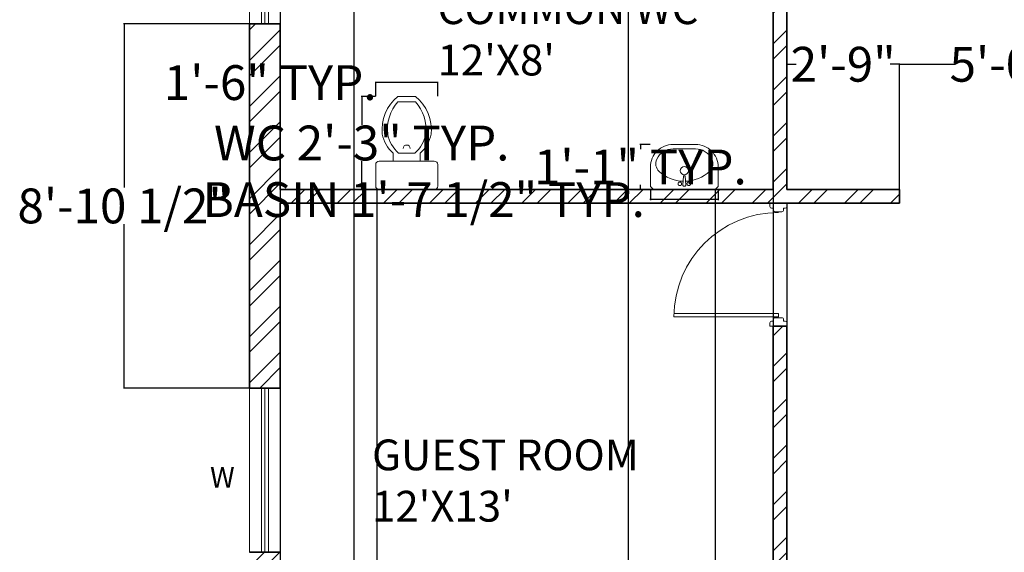
# Model space of a CAD drawing. Units: inches. Extents: x 1583 to 2239, y 1430 to 2174.
# Tile 2 of 5: x 1583 to 1871, y 1588 to 1743. Entities that reach past the tile are written whole.
import ezdxf

# ---------------------------------------------------------------- set-up
doc = ezdxf.new("R2010")
doc.units = ezdxf.units.IN
doc.linetypes.add('ACAD_ISO02W100', pattern=[15, 12, -3])
for name, color, linetype, lineweight in [('00 FURNITURE', 15, 'Continuous', 15), ('A-ANNO-DIMS', 2, 'Continuous', 18), ('A-ANNO-TEXT', 7, 'Continuous', 18), ('A-AREA-IDEN', 7, 'Continuous', 25), ('A-DOOR', 3, 'Continuous', 18), ('A-FLOR-FIXT', 9, 'Continuous', 18), ('A-GLAZ-VENT', 6, 'ACAD_ISO02W100', 13), ('A-WALL-PATT', 252, 'Continuous', 13), ('WALL', 7, 'Continuous', 35), ('WINDOW', 160, 'Continuous', 18)]:
    doc.layers.add(name, color=color, linetype=linetype, lineweight=lineweight)
doc.styles.get("Standard").update_dxf_attribs({"font": 'arial.ttf'})
doc.dimstyles.get("Standard").update_dxf_attribs({"dimtxt": 10.18, "dimasz": 0.18, "dimexe": 0.18, "dimexo": 0.0625, "dimgap": 0.09, "dimtad": 0, "dimtih": 1, "dimtoh": 1, "dimdec": 0, "dimzin": 0, "dimdsep": 46, "dimlunit": 3, "dimtxsty": 'Standard', "dimcen": 0.09, "dimadec": 0, "dimazin": 0, "dimtfac": 1, "dimtdec": 0, "dimtofl": 0, "dimtmove": 0, "dimatfit": 3, "dimfxl": 1, "dimtolj": 1, "dimtzin": 0, "dimarcsym": 0})

# ---------------------------------------------------------------- blocks, each defined once
blk = doc.blocks.new('DDD')
at = {"layer": '00 FURNITURE'}
for p, q in [((-12579.77, -15859.53), (-12579.77, -15829.05)), ((-12578.77, -15859.53), (-12578.77, -15829.03)), ((-12612.02, -15857.03), (-12612.02, -15862.03)), ((-12611.02, -15857.03), (-12612.02, -15857.03)), ((-12577.02, -15857.03), (-12576.02, -15857.03)), ((-12576.02, -15857.03), (-12576.02, -15862.03)), ((-12610.52, -15858.03), (-12610.52, -15857.53)), ((-12578.77, -15859.53), (-12579.77, -15859.53)), ((-12577.52, -15858.03), (-12577.52, -15857.53)), ((-12612.02, -15862.03), (-12611.02, -15862.03)), ((-12610.52, -15861.53), (-12610.52, -15861.03)), ((-12577.52, -15861.53), (-12577.52, -15861.03)), ((-12576.02, -15862.03), (-12577.02, -15862.03))]:
    blk.add_line(p, q, dxfattribs=at)
for points in [[(-12610.52, -15861.03), (-12610.02, -15861.03, 0.414214), (-12609.52, -15860.53), (-12609.52, -15858.53, 0.414214), (-12610.02, -15858.03), (-12610.52, -15858.03)], [(-12577.52, -15861.03), (-12578.02, -15861.03, -0.414214), (-12578.52, -15860.53), (-12578.52, -15858.53, -0.414214), (-12578.02, -15858.03), (-12577.52, -15858.03)]]:
    blk.add_lwpolyline(points, format="xyb", dxfattribs=at)
for centre, radius, start, end in [((-12578.77, -15859.53), 30.5, 90, 180), ((-12611.02, -15857.53), 0.5, 0, 90), ((-12577.02, -15857.53), 0.5, 90, 180), ((-12611.02, -15861.53), 0.5, 270, 0), ((-12577.02, -15861.53), 0.5, 180, 270)]:
    blk.add_arc(centre, radius, start, end, dxfattribs=at)
blk = doc.blocks.new('A$C2AC94788')
for p, q in [((0, 0.505), (0, 0.665)), ((0.025, 0.69), (0.435, 0.69)), ((0.46, 0.665), (0.46, 0.505)), ((0.435, 0.48), (0.025, 0.48)), ((0.13, 0.48), (0.13, 0.42)), ((0.33, 0.42), (0.33, 0.48)), ((0.17, 0.42), (0.29, 0.42)), ((0.1641, 0.0392), (0.2959, 0.0392)), ((0.2291, 0.0392), (0.23, 0.0392)), ((0.2309, 0.0392), (0.23, 0.0392)), ((0.165, 0), (0.295, 0))]:
    blk.add_line(p, q)
for centre, radius, start, end in [((0.025, 0.665), 0.025, 90, 180), ((0.435, 0.665), 0.025, 0, 90), ((0.025, 0.505), 0.025, 180, 270), ((0.435, 0.505), 0.025, 270, 0), ((0.2874, 0.2356), 0.2425, 130.48854, 169.44501), ((0.3274, 0.2356), 0.2425, 130.48854, 169.44501), ((0.23, 0.385), 0.025, 180, 0), ((0.1326, 0.2356), 0.2425, 10.55499, 49.51146), ((0.1726, 0.2356), 0.2425, 10.55499, 49.51146), ((0.3601, 0.2448), 0.313, 173.53688, 231.44828), ((0.4001, 0.2448), 0.313, 173.53688, 221.06038), ((0.0999, 0.2448), 0.313, 308.55172, 6.46312), ((0.0599, 0.2448), 0.313, 318.93962, 6.46312)]:
    blk.add_arc(centre, radius, start, end)
blk = doc.blocks.new('s_46')
at = {"ltscale": 600}
h = blk.add_hatch(color=256, dxfattribs=at)
edge = h.paths.add_edge_path()
edge.add_line((13.5, 62), (14.2, 54.1))
edge.add_ellipse((4.2, 52.3), major_axis=(-10.1, 0), ratio=1, start_angle=540, end_angle=550.17546, ccw=False)
edge.add_arc((4.2, 52.3), 10.1, 270, 360, ccw=False)
edge.add_line((4.2, 42.2), (4.2, 41.3))
edge.add_line((4.2, 41.3), (11.9, 41.3))
edge.add_arc((4.2, 52.3), 13.4, 664.69813, 766.48477)
h.paths.add_polyline_path([(4.2, 41.3), (-3.4, 41.3, 0.152567), (4.2, 38.9)])
h.paths.add_polyline_path([(11.9, 41.3), (4.2, 41.3), (4.2, 38.9, 0.152567)])
h.paths.add_polyline_path([(-5.7, 54.1), (-5, 62, 0.475833), (-3.4, 41.3), (4.2, 41.3), (4.2, 42.2, -0.46724)])
for p, q in [((-5.9, 52.3), (-0.7, 110.5)), ((-5.9, 52.3), (-0.7, 110.5)), ((9.1, 110.5), (14.2, 54.1)), ((14.3, 52.3), (9.1, 110.5)), ((14.2, 54.1), (14.3, 52.3))]:
    blk.add_line(p, q, dxfattribs=at)
blk.add_lwpolyline([(-220.8, 171.3, -0.414214), (-70.8, 321.3), (79.2, 321.3, -0.414214), (229.2, 171.3), (229.2, 41.3), (209.2, 21.3), (-200.8, 21.3), (-220.8, 41.3)], format="xyb", close=True, dxfattribs=at)
blk.add_lwpolyline([(12.3, 75.4, 0.181638), (172.2, 141.5, 0.326351), (187.7, 222.7, 0.289814), (79.2, 291.3), (-70.8, 291.3, 0.289814), (-179.2, 222.7, 0.326351), (-163.8, 141.5, 0.181638), (-3.8, 75.4)], format="xyb", dxfattribs=at)
for points in [[(-16.8, 67.4), (-17, 67.5), (-17.2, 67.6), (-17.4, 67.6), (-17.6, 67.7), (-17.8, 67.8), (-18, 67.9), (-18.1, 68.1), (-18.2, 68.2), (-18.3, 68.4), (-18.4, 68.6), (-18.5, 68.8), (-18.7, 68.9), (-18.8, 69.1), (-18.9, 69.2), (-19.1, 69.3), (-19.3, 69.3), (-19.5, 69.3), (-19.7, 69.4), (-19.9, 69.4), (-20.1, 69.4), (-20.3, 69.4), (-20.5, 69.5), (-20.7, 69.6), (-20.8, 69.7), (-21, 69.9), (-21.1, 70), (-21.3, 70.2), (-21.4, 70.3), (-21.5, 70.4), (-21.7, 70.5), (-21.9, 70.5), (-22.1, 70.5), (-22.3, 70.5), (-22.5, 70.5), (-22.7, 70.4), (-22.9, 70.4), (-23.1, 70.4), (-23.3, 70.4), (-23.5, 70.5), (-23.7, 70.6), (-23.9, 70.7), (-24, 70.8), (-24.2, 70.9), (-24.4, 71), (-24.6, 71.1), (-24.7, 71.1), (-24.9, 71.1), (-25.1, 71), (-25.3, 71), (-25.5, 70.9), (-25.7, 70.8), (-25.9, 70.7), (-26.1, 70.6), (-26.3, 70.6), (-26.5, 70.6), (-26.7, 70.6), (-26.9, 70.7), (-27.1, 70.8), (-27.3, 70.8), (-27.5, 70.9), (-27.7, 70.9), (-27.8, 70.9), (-28, 70.8), (-28.2, 70.8), (-28.3, 70.6), (-28.5, 70.5), (-28.7, 70.4), (-28.9, 70.3), (-29.1, 70.2), (-29.3, 70.1), (-29.6, 70.1), (-29.9, 70.1), (-30.2, 70.1), (-30.5, 70), (-30.8, 69.8), (-31.1, 69.5), (-31.4, 69), (-31.6, 68.4), (-32.3, 68.5), (-32.8, 68.4), (-33.2, 68.3), (-33.5, 68.1), (-33.7, 67.8), (-33.9, 67.6), (-34, 67.3), (-34.1, 67.1), (-34.3, 66.9), (-34.5, 66.7), (-34.7, 66.6), (-34.9, 66.5), (-35.1, 66.4), (-35.2, 66.3), (-35.4, 66.2), (-35.5, 66), (-35.6, 65.9), (-35.6, 65.7), (-35.7, 65.5), (-35.7, 65.3), (-35.7, 65.1), (-35.8, 64.9), (-35.8, 64.7), (-35.9, 64.5), (-36, 64.3), (-36.2, 64.2), (-36.3, 64), (-36.5, 63.9), (-36.6, 63.8), (-36.8, 63.6), (-36.9, 63.5), (-37, 63.3), (-37, 63.1), (-37, 63), (-37, 62.8), (-37, 62.6), (-37, 62.3), (-37, 62.1), (-37, 61.9), (-37, 61.7), (-37.1, 61.5), (-37.2, 61.4), (-37.3, 61.2), (-37.4, 61), (-37.5, 60.8), (-37.6, 60.7), (-37.7, 60.5), (-37.8, 60.3), (-37.8, 60.1), (-37.7, 60), (-37.7, 59.8), (-37.6, 59.6), (-37.5, 59.4), (-37.4, 59.2), (-37.4, 59), (-37.4, 58.8), (-37.4, 58.6), (-37.4, 58.4), (-37.5, 58.2), (-37.6, 58), (-37.7, 57.8), (-37.7, 57.6), (-37.8, 57.4), (-37.8, 57.2), (-37.7, 57.1), (-37.6, 56.9), (-37.5, 56.7), (-37.4, 56.6), (-37.3, 56.4), (-37.2, 56.2), (-37.1, 56), (-37, 55.8), (-37, 55.6), (-37, 55.4), (-37, 55.2), (-37, 55), (-37, 54.8), (-37, 54.6), (-37, 54.4), (-37, 54.2), (-36.9, 54.1), (-36.8, 53.9), (-36.6, 53.8), (-36.5, 53.7), (-36.3, 53.5), (-36.2, 53.4), (-36, 53.2), (-35.9, 53.1), (-35.8, 52.9), (-35.8, 52.7), (-35.7, 52.5), (-35.7, 52.3), (-35.7, 52.1), (-35.6, 51.9), (-35.6, 51.7), (-35.5, 51.5), (-35.4, 51.4), (-35.2, 51.3), (-35.1, 51.2), (-34.9, 51.1), (-34.7, 51), (-34.5, 50.9), (-34.3, 50.8), (-34.2, 50.7), (-34, 50.5), (-33.9, 50.3), (-33.8, 50.1), (-33.8, 49.9), (-33.7, 49.8), (-33.6, 49.6), (-33.5, 49.4), (-33.4, 49.3), (-33.2, 49.2), (-33.1, 49.1), (-32.9, 49.1), (-32.7, 49), (-32.5, 49), (-32.2, 48.9), (-32.1, 48.9), (-31.9, 48.8), (-31.7, 48.7), (-31.6, 48.5), (-31.4, 48.3), (-31.3, 48.2), (-31.2, 48), (-31.1, 47.9), (-30.9, 47.7), (-30.8, 47.6), (-30.6, 47.6), (-30.4, 47.5), (-30.2, 47.5), (-30, 47.6), (-29.8, 47.6), (-29.6, 47.6), (-29.4, 47.6), (-29.2, 47.5), (-29, 47.4), (-28.8, 47.3), (-28.7, 47.2), (-28.5, 47.1), (-28.3, 46.9), (-28.2, 46.8), (-28, 46.7), (-27.8, 46.7), (-27.7, 46.7), (-27.5, 46.7), (-27.3, 46.7), (-27.1, 46.8), (-26.9, 46.9), (-26.7, 46.9), (-26.5, 47), (-26.3, 47), (-26.1, 46.9), (-25.9, 46.9), (-25.7, 46.8), (-25.5, 46.7), (-25.3, 46.6), (-25.1, 46.5), (-24.9, 46.5), (-24.7, 46.5), (-24.6, 46.5), (-24.4, 46.6), (-24.2, 46.7), (-24, 46.8), (-23.9, 46.9), (-23.7, 47), (-23.5, 47.1), (-23.3, 47.1), (-23.1, 47.2), (-22.9, 47.2), (-22.7, 47.1), (-22.5, 47.1), (-22.3, 47), (-22.1, 47), (-21.9, 47), (-21.7, 47.1), (-21.5, 47.1), (-21.4, 47.2), (-21.3, 47.4), (-21.1, 47.5), (-21, 47.7), (-20.8, 47.8), (-20.7, 48), (-20.5, 48.1), (-20.3, 48.1), (-20.1, 48.2), (-19.9, 48.2), (-19.7, 48.2), (-19.5, 48.2), (-19.3, 48.2), (-19.1, 48.3), (-18.9, 48.4), (-18.8, 48.5), (-18.7, 48.6), (-18.5, 48.8), (-18.4, 49), (-18.3, 49.2), (-18.2, 49.3), (-18.1, 49.5), (-18, 49.7), (-17.8, 49.8), (-17.6, 49.9), (-17.4, 49.9), (-17.2, 50), (-17, 50.1), (-16.8, 50.1), (-16.7, 50.2), (-16.5, 50.3), (-16.4, 50.5), (-16.3, 50.7), (-16.3, 50.8), (-16.2, 51), (-16.2, 51.3), (-16.1, 51.5), (-16, 51.6), (-15.9, 51.8), (-15.8, 52), (-15.6, 52.1), (-15.5, 52.2), (-15.3, 52.3), (-15.1, 52.4), (-15, 52.6), (-14.8, 52.7), (-14.7, 52.8), (-14.7, 53), (-14.6, 53.2), (-14.6, 53.4), (-14.6, 53.6), (-14.6, 53.8), (-14.6, 54), (-14.6, 54.2), (-14.5, 54.4), (-14.4, 54.6), (-14.3, 54.8), (-14.2, 54.9), (-14, 55.1), (-13.9, 55.2), (-13.7, 55.4), (-13.6, 55.5), (-13.6, 55.7), (-13.6, 55.9), (-13.6, 56.1), (-13.6, 56.3), (-13.7, 56.5), (-13.7, 56.7), (-13.8, 56.9), (-13.8, 57.1), (-13.8, 57.3), (-13.7, 57.5), (-13.7, 57.7), (-13.6, 57.9), (-13.5, 58.1), (-13.4, 58.2), (-13.3, 58.4), (-13.2, 58.6), (-13.2, 58.8), (-13.2, 59), (-13.3, 59.1), (-13.4, 59.3), (-13.5, 59.5), (-13.6, 59.7), (-13.7, 59.9), (-13.7, 60.1), (-13.8, 60.3), (-13.8, 60.5), (-13.8, 60.7), (-13.7, 60.9), (-13.7, 61.1), (-13.6, 61.3), (-13.6, 61.5), (-13.6, 61.7), (-13.6, 61.9), (-13.6, 62), (-13.7, 62.2), (-13.9, 62.3), (-14, 62.5), (-14.2, 62.6), (-14.3, 62.8), (-14.4, 63), (-14.5, 63.1), (-14.6, 63.3), (-14.6, 63.5), (-14.6, 63.8), (-14.6, 64), (-14.6, 64.2), (-14.6, 64.4), (-14.7, 64.6), (-14.7, 64.7), (-14.8, 64.9), (-15, 65), (-15.1, 65.1), (-15.3, 65.2), (-15.5, 65.3), (-15.6, 65.5), (-15.8, 65.6), (-15.9, 65.7), (-16, 65.9), (-16.1, 66.1), (-16.2, 66.3), (-16.2, 66.5), (-16.3, 66.7), (-16.3, 66.9), (-16.4, 67.1), (-16.5, 67.2), (-16.7, 67.3)], [(22.1, 61.1), (22, 61.3), (22, 61.5), (22, 61.7), (22, 61.9), (22.1, 62), (22.2, 62.2), (22.3, 62.3), (22.4, 62.5), (22.6, 62.6), (22.7, 62.8), (22.8, 63), (22.9, 63.1), (23, 63.3), (23, 63.5), (23, 63.8), (23, 64), (23, 64.2), (23, 64.4), (23.1, 64.6), (23.1, 64.7), (23.2, 64.9), (23.4, 65), (23.5, 65.1), (23.7, 65.2), (23.9, 65.3), (24.1, 65.5), (24.2, 65.6), (24.4, 65.7), (24.5, 65.9), (24.5, 66.1), (24.6, 66.3), (24.7, 66.5), (24.7, 66.7), (24.8, 66.9), (24.9, 67.1), (25, 67.2), (25.1, 67.3), (25.3, 67.4), (25.4, 67.5), (25.6, 67.6), (25.8, 67.6), (26, 67.7), (26.2, 67.8), (26.4, 67.9), (26.5, 68.1), (26.7, 68.2), (26.8, 68.4), (26.9, 68.6), (27, 68.8), (27.1, 68.9), (27.2, 69.1), (27.3, 69.2), (27.5, 69.3), (27.7, 69.3), (27.9, 69.3), (28.1, 69.4), (28.3, 69.4), (28.5, 69.4), (28.7, 69.4), (28.9, 69.5), (29.1, 69.6), (29.2, 69.7), (29.4, 69.9), (29.5, 70), (29.7, 70.2), (29.8, 70.3), (30, 70.4), (30.1, 70.5), (30.3, 70.5), (30.5, 70.5), (30.7, 70.5), (30.9, 70.5), (31.1, 70.4), (31.3, 70.4), (31.5, 70.4), (31.7, 70.4), (31.9, 70.5), (32.1, 70.6), (32.3, 70.7), (32.5, 70.8), (32.6, 70.9), (32.8, 71), (33, 71.1), (33.2, 71.1), (33.4, 71.1), (33.5, 71), (33.7, 71), (33.9, 70.9), (34.1, 70.8), (34.3, 70.7), (34.5, 70.6), (34.7, 70.6), (34.9, 70.6), (35.1, 70.6), (35.3, 70.7), (35.5, 70.8), (35.7, 70.8), (35.9, 70.9), (36.1, 70.9), (36.3, 70.9), (36.4, 70.8), (36.6, 70.8), (36.8, 70.6), (36.9, 70.5), (37.1, 70.4), (37.3, 70.3), (37.5, 70.2), (37.8, 70.1), (38, 70.1), (38.3, 70.1), (38.6, 70.1), (38.9, 70), (39.2, 69.8), (39.5, 69.5), (39.8, 69), (40.1, 68.4), (40.7, 68.5), (41.3, 68.4), (41.7, 68.3), (42, 68.1), (42.2, 67.8), (42.3, 67.6), (42.4, 67.3), (42.6, 67.1), (42.7, 66.9), (42.9, 66.7), (43.1, 66.6), (43.3, 66.5), (43.5, 66.4), (43.6, 66.3), (43.8, 66.2), (43.9, 66), (44, 65.9), (44.1, 65.7), (44.1, 65.5), (44.1, 65.3), (44.2, 65.1), (44.2, 64.9), (44.2, 64.7), (44.3, 64.5), (44.4, 64.3), (44.6, 64.2), (44.7, 64), (44.9, 63.9), (45.1, 63.8), (45.2, 63.6), (45.3, 63.5), (45.4, 63.3), (45.5, 63.1), (45.5, 63), (45.5, 62.8), (45.4, 62.6), (45.4, 62.3), (45.4, 62.1), (45.4, 61.9), (45.4, 61.7), (45.5, 61.5), (45.6, 61.4), (45.7, 61.2), (45.8, 61), (46, 60.8), (46.1, 60.7), (46.1, 60.5), (46.2, 60.3), (46.2, 60.1), (46.1, 60), (46.1, 59.8), (46, 59.6), (45.9, 59.4), (45.9, 59.2), (45.8, 59), (45.8, 58.8), (45.8, 58.6), (45.9, 58.4), (45.9, 58.2), (46, 58), (46.1, 57.8), (46.1, 57.6), (46.2, 57.4), (46.2, 57.2), (46.1, 57.1), (46.1, 56.9), (46, 56.7), (45.8, 56.6), (45.7, 56.4), (45.6, 56.2), (45.5, 56), (45.4, 55.8), (45.4, 55.6), (45.4, 55.4), (45.4, 55.2), (45.4, 55), (45.5, 54.8), (45.5, 54.6), (45.5, 54.4), (45.4, 54.2), (45.3, 54.1), (45.2, 53.9), (45.1, 53.8), (44.9, 53.7), (44.7, 53.5), (44.6, 53.4), (44.4, 53.2), (44.3, 53.1), (44.2, 52.9), (44.2, 52.7), (44.2, 52.5), (44.1, 52.3), (44.1, 52.1), (44.1, 51.9), (44, 51.7), (43.9, 51.5), (43.8, 51.4), (43.6, 51.3), (43.5, 51.2), (43.3, 51.1), (43.1, 51), (42.9, 50.9), (42.7, 50.8), (42.6, 50.7), (42.5, 50.5), (42.4, 50.3), (42.3, 50.1), (42.2, 49.9), (42.1, 49.8), (42, 49.6), (41.9, 49.4), (41.8, 49.3), (41.7, 49.2), (41.5, 49.1), (41.3, 49.1), (41.1, 49), (40.9, 49), (40.7, 48.9), (40.5, 48.9), (40.3, 48.8), (40.1, 48.7), (40, 48.5), (39.9, 48.3), (39.7, 48.2), (39.6, 48), (39.5, 47.9), (39.4, 47.7), (39.2, 47.6), (39, 47.6), (38.8, 47.5), (38.6, 47.5), (38.4, 47.6), (38.2, 47.6), (38, 47.6), (37.8, 47.6), (37.6, 47.5), (37.4, 47.4), (37.2, 47.3), (37.1, 47.2), (36.9, 47.1), (36.8, 46.9), (36.6, 46.8), (36.4, 46.7), (36.3, 46.7), (36.1, 46.7), (35.9, 46.7), (35.7, 46.7), (35.5, 46.8), (35.3, 46.9), (35.1, 46.9), (34.9, 47), (34.7, 47), (34.5, 46.9), (34.3, 46.9), (34.1, 46.8), (33.9, 46.7), (33.7, 46.6), (33.5, 46.5), (33.4, 46.5), (33.2, 46.5), (33, 46.5), (32.8, 46.6), (32.6, 46.7), (32.5, 46.8), (32.3, 46.9), (32.1, 47), (31.9, 47.1), (31.7, 47.1), (31.5, 47.2), (31.3, 47.2), (31.1, 47.1), (30.9, 47.1), (30.7, 47), (30.5, 47), (30.3, 47), (30.1, 47.1), (30, 47.1), (29.8, 47.2), (29.7, 47.4), (29.5, 47.5), (29.4, 47.7), (29.2, 47.8), (29.1, 48), (28.9, 48.1), (28.7, 48.1), (28.5, 48.2), (28.3, 48.2), (28.1, 48.2), (27.9, 48.2), (27.7, 48.2), (27.5, 48.3), (27.3, 48.4), (27.2, 48.5), (27.1, 48.6), (27, 48.8), (26.9, 49), (26.8, 49.2), (26.7, 49.3), (26.5, 49.5), (26.4, 49.7), (26.2, 49.8), (26, 49.9), (25.8, 49.9), (25.6, 50), (25.4, 50.1), (25.3, 50.1), (25.1, 50.2), (25, 50.3), (24.9, 50.5), (24.8, 50.7), (24.7, 50.8), (24.7, 51), (24.6, 51.3), (24.5, 51.5), (24.5, 51.6), (24.4, 51.8), (24.2, 52), (24.1, 52.1), (23.9, 52.2), (23.7, 52.3), (23.5, 52.4), (23.4, 52.6), (23.2, 52.7), (23.1, 52.8), (23.1, 53), (23, 53.2), (23, 53.4), (23, 53.6), (23, 53.8), (23, 54), (23, 54.2), (22.9, 54.4), (22.8, 54.6), (22.7, 54.8), (22.6, 54.9), (22.4, 55.1), (22.3, 55.2), (22.2, 55.4), (22.1, 55.5), (22, 55.7), (22, 55.9), (22, 56.1), (22, 56.3), (22.1, 56.5), (22.1, 56.7), (22.2, 56.9), (22.2, 57.1), (22.2, 57.3), (22.2, 57.5), (22.1, 57.7), (22, 57.9), (21.9, 58.1), (21.8, 58.2), (21.7, 58.4), (21.6, 58.6), (21.6, 58.8), (21.6, 59), (21.7, 59.1), (21.8, 59.3), (21.9, 59.5), (22, 59.7), (22.1, 59.9), (22.2, 60.1), (22.2, 60.3), (22.2, 60.5), (22.2, 60.7), (22.1, 60.9)]]:
    blk.add_lwpolyline(points, close=True, dxfattribs=at)
blk.add_circle((4.2, 146.3), 28, dxfattribs=at)
for centre, radius, start, end in [((4.2, 108.2), 5.42, 24.6783, 155.3217), ((4.2, 52.3), 10.1, 169.82454, 0)]:
    blk.add_arc(centre, radius, start, end, dxfattribs=at)
for centre, major_axis, ratio, start_param, end_param in [((4.2, 110.5), (-4.93, 0), 0.641024, 3.141593, 6.283185), ((4.2, 52.3), (-10.1, 0), 1, 6.10559, 9.602373)]:
    blk.add_ellipse(centre, major_axis=major_axis, ratio=ratio, start_param=start_param, end_param=end_param, dxfattribs=at)
blk = doc.blocks.new('WIN-SASH-48IN')
for p, q in [((48, 2), (0, 2)), ((48, 1), (0, 1)), ((48, 0), (0, 0))]:
    blk.add_line(p, q)
blk = doc.blocks.new('VENT-GRILLE-24IN')
for p, q in [((24, 2), (0, 2)), ((24, 1), (0, 1)), ((24, 0), (0, 0))]:
    blk.add_line(p, q)
blk = doc.blocks.new('*D21')
at = {"layer": 'A-ANNO-DIMS', "color": 0, "lineweight": -2, "transparency": 16777216}
for p, q in [((1767.67, 1693.58), (1767.67, 1690.5)), ((1787.42, 1693.58), (1787.42, 1690.5)), ((1767.67, 1690.68), (1767.49, 1690.68)), ((1787.24, 1690.68), (1767.85, 1690.68))]:
    blk.add_line(p, q, dxfattribs=at)
at = {"layer": 'A-ANNO-DIMS', "color": 0, "transparency": 16777216}
for points in [[(1767.85, 1690.71), (1767.85, 1690.65), (1767.67, 1690.68)], [(1787.24, 1690.71), (1787.24, 1690.65), (1787.42, 1690.68)]]:
    blk.add_solid(points, dxfattribs=at)
at = {"layer": 'Defpoints', "color": 0, "transparency": 16777216}
for p in [(1767.67, 1693.64), (1787.42, 1693.64), (1767.67, 1690.68)]:
    blk.add_point(p, dxfattribs=at)
at = {"layer": 'A-ANNO-DIMS', "color": 0, "transparency": 16777216, "insert": (1701.43, 1690.68), "char_height": 10.18, "attachment_point": 5}
blk.add_mtext('\\A1;BASIN 1\'-7 1/2" TYP.', dxfattribs=at)
blk = doc.blocks.new('*D22')
at = {"layer": 'A-ANNO-DIMS', "color": 0, "lineweight": -2, "transparency": 16777216}
for p, q in [((1767.61, 1706.8), (1764.53, 1706.8)), ((1764.71, 1706.62), (1764.71, 1705.43)), ((1764.71, 1693.82), (1764.71, 1695.02)), ((1767.61, 1693.64), (1764.53, 1693.64))]:
    blk.add_line(p, q, dxfattribs=at)
at = {"layer": 'A-ANNO-DIMS', "color": 0, "transparency": 16777216}
for points in [[(1764.68, 1706.62), (1764.74, 1706.62), (1764.71, 1706.8)], [(1764.68, 1693.82), (1764.74, 1693.82), (1764.71, 1693.64)]]:
    blk.add_solid(points, dxfattribs=at)
at = {"layer": 'Defpoints', "color": 0, "transparency": 16777216}
for p in [(1764.71, 1706.8), (1767.67, 1706.8), (1767.67, 1693.64)]:
    blk.add_point(p, dxfattribs=at)
at = {"layer": 'A-ANNO-DIMS', "color": 0, "transparency": 16777216, "insert": (1764.71, 1700.22), "char_height": 10.18, "attachment_point": 5}
blk.add_mtext('\\A1;1\'-1" TYP.', dxfattribs=at)
blk = doc.blocks.new('*D23')
at = {"layer": 'A-ANNO-DIMS', "color": 0, "lineweight": -2, "transparency": 16777216}
for p, q in [((1687.33, 1720.81), (1683.13, 1720.81)), ((1683.31, 1720.63), (1683.31, 1712.58)), ((1683.31, 1693.82), (1683.31, 1701.87)), ((1687.33, 1693.64), (1683.13, 1693.64))]:
    blk.add_line(p, q, dxfattribs=at)
at = {"layer": 'A-ANNO-DIMS', "color": 0, "transparency": 16777216}
for points in [[(1683.28, 1720.63), (1683.34, 1720.63), (1683.31, 1720.81)], [(1683.28, 1693.82), (1683.34, 1693.82), (1683.31, 1693.64)]]:
    blk.add_solid(points, dxfattribs=at)
at = {"layer": 'Defpoints', "color": 0, "transparency": 16777216}
for p in [(1687.39, 1720.81), (1683.31, 1693.64), (1687.39, 1693.64)]:
    blk.add_point(p, dxfattribs=at)
at = {"layer": 'A-ANNO-DIMS', "color": 0, "transparency": 16777216, "insert": (1683.31, 1707.22), "char_height": 10.18, "attachment_point": 5}
blk.add_mtext('\\A1;WC 2\'-3" TYP.', dxfattribs=at)
blk = doc.blocks.new('*D24')
at = {"layer": 'A-ANNO-DIMS', "color": 0, "lineweight": -2, "transparency": 16777216}
for p, q in [((1687.39, 1724.88), (1687.21, 1724.88)), ((1687.39, 1720.87), (1687.39, 1725.06)), ((1705.32, 1724.88), (1687.57, 1724.88)), ((1705.5, 1720.87), (1705.5, 1725.06))]:
    blk.add_line(p, q, dxfattribs=at)
at = {"layer": 'A-ANNO-DIMS', "color": 0, "transparency": 16777216}
for points in [[(1687.57, 1724.91), (1687.57, 1724.85), (1687.39, 1724.88)], [(1705.32, 1724.91), (1705.32, 1724.85), (1705.5, 1724.88)]]:
    blk.add_solid(points, dxfattribs=at)
at = {"layer": 'Defpoints', "color": 0, "transparency": 16777216}
for p in [(1687.39, 1724.88), (1687.39, 1720.81), (1705.5, 1720.81)]:
    blk.add_point(p, dxfattribs=at)
at = {"layer": 'A-ANNO-DIMS', "color": 0, "transparency": 16777216, "insert": (1656.57, 1724.88), "char_height": 10.18, "attachment_point": 5}
blk.add_mtext('\\A1;1\'-6" TYP.', dxfattribs=at)
blk = doc.blocks.new('*D37')
at = {"layer": 'A-ANNO-DIMS', "color": 0, "lineweight": -2, "transparency": 16777216}
for p, q in [((1650.47, 1742.08), (1613.75, 1742.08)), ((1613.93, 1741.9), (1613.93, 1694.17)), ((1613.93, 1635.74), (1613.93, 1683.46)), ((1650.47, 1635.56), (1613.75, 1635.56))]:
    blk.add_line(p, q, dxfattribs=at)
at = {"layer": 'A-ANNO-DIMS', "color": 0, "transparency": 16777216}
for points in [[(1613.9, 1741.9), (1613.96, 1741.9), (1613.93, 1742.08)], [(1613.9, 1635.74), (1613.96, 1635.74), (1613.93, 1635.56)]]:
    blk.add_solid(points, dxfattribs=at)
at = {"layer": 'Defpoints', "color": 0, "transparency": 16777216}
for p in [(1613.93, 1742.08), (1650.53, 1742.08), (1650.53, 1635.56)]:
    blk.add_point(p, dxfattribs=at)
at = {"layer": 'A-ANNO-DIMS', "color": 0, "transparency": 16777216, "insert": (1613.93, 1688.82), "char_height": 10.18, "attachment_point": 5}
blk.add_mtext('\\A1;8\'-10 1/2"', dxfattribs=at)
blk = doc.blocks.new('*D49')
at = {"layer": 'A-ANNO-DIMS', "color": 0, "lineweight": -2, "transparency": 16777216}
for p, q in [((1803.53, 1693.58), (1803.53, 1485.86)), ((1807.53, 1689.58), (1807.53, 1485.86)), ((1803.71, 1486.04), (1807.35, 1486.04)), ((1807.53, 1486.04), (1807.71, 1486.04))]:
    blk.add_line(p, q, dxfattribs=at)
at = {"layer": 'A-ANNO-DIMS', "color": 0, "transparency": 16777216}
for points in [[(1803.71, 1486.07), (1803.71, 1486.01), (1803.53, 1486.04)], [(1807.35, 1486.07), (1807.35, 1486.01), (1807.53, 1486.04)]]:
    blk.add_solid(points, dxfattribs=at)
at = {"layer": 'Defpoints', "color": 0, "transparency": 16777216}
for p in [(1803.53, 1693.64), (1807.53, 1689.64), (1807.53, 1486.04)]:
    blk.add_point(p, dxfattribs=at)
at = {"layer": 'A-ANNO-DIMS', "color": 0, "transparency": 16777216, "insert": (1821.33, 1486.04), "char_height": 10.18, "attachment_point": 5}
blk.add_mtext('\\A1;0\'-4"', dxfattribs=at)
blk = doc.blocks.new('*D51')
at = {"layer": 'A-ANNO-DIMS', "color": 0, "lineweight": -2, "transparency": 16777216}
for p, q in [((1840.39, 1693.7), (1840.39, 1730.42)), ((1840.57, 1730.24), (1856.77, 1730.24)), ((1900.21, 1730.24), (1884.01, 1730.24)), ((1900.39, 1693.7), (1900.39, 1730.42))]:
    blk.add_line(p, q, dxfattribs=at)
at = {"layer": 'A-ANNO-DIMS', "color": 0, "transparency": 16777216}
for points in [[(1840.57, 1730.27), (1840.57, 1730.21), (1840.39, 1730.24)], [(1900.21, 1730.27), (1900.21, 1730.21), (1900.39, 1730.24)]]:
    blk.add_solid(points, dxfattribs=at)
at = {"layer": 'Defpoints', "color": 0, "transparency": 16777216}
for p in [(1900.39, 1730.24), (1840.39, 1693.64), (1900.39, 1693.64)]:
    blk.add_point(p, dxfattribs=at)
at = {"layer": 'A-ANNO-DIMS', "color": 0, "transparency": 16777216, "insert": (1870.39, 1730.24), "char_height": 10.18, "attachment_point": 5}
blk.add_mtext('\\A1;5\'-0"', dxfattribs=at)
blk = doc.blocks.new('*D52')
at = {"layer": 'A-ANNO-DIMS', "color": 0, "lineweight": -2, "transparency": 16777216}
for p, q in [((1807.53, 1693.7), (1807.53, 1730.42)), ((1807.71, 1730.24), (1810.25, 1730.24)), ((1840.21, 1730.24), (1837.67, 1730.24)), ((1840.39, 1693.7), (1840.39, 1730.42))]:
    blk.add_line(p, q, dxfattribs=at)
at = {"layer": 'A-ANNO-DIMS', "color": 0, "transparency": 16777216}
for points in [[(1807.71, 1730.27), (1807.71, 1730.21), (1807.53, 1730.24)], [(1840.21, 1730.27), (1840.21, 1730.21), (1840.39, 1730.24)]]:
    blk.add_solid(points, dxfattribs=at)
at = {"layer": 'Defpoints', "color": 0, "transparency": 16777216}
for p in [(1840.39, 1730.24), (1807.53, 1693.64), (1840.39, 1693.64)]:
    blk.add_point(p, dxfattribs=at)
at = {"layer": 'A-ANNO-DIMS', "color": 0, "transparency": 16777216, "insert": (1823.96, 1730.24), "char_height": 10.18, "attachment_point": 5}
blk.add_mtext('\\A1;2\'-9"', dxfattribs=at)
blk = doc.blocks.new('*D53')
at = {"layer": 'A-ANNO-DIMS', "color": 0, "lineweight": -2, "transparency": 16777216}
for p, q in [((1659.53, 1693.58), (1659.53, 1485.86)), ((1687.68, 1693.86), (1687.68, 1485.86)), ((1659.71, 1486.04), (1659.9, 1486.04)), ((1687.5, 1486.04), (1687.31, 1486.04))]:
    blk.add_line(p, q, dxfattribs=at)
at = {"layer": 'A-ANNO-DIMS', "color": 0, "transparency": 16777216}
for points in [[(1659.71, 1486.07), (1659.71, 1486.01), (1659.53, 1486.04)], [(1687.5, 1486.07), (1687.5, 1486.01), (1687.68, 1486.04)]]:
    blk.add_solid(points, dxfattribs=at)
at = {"layer": 'Defpoints', "color": 0, "transparency": 16777216}
for p in [(1659.53, 1693.64), (1687.68, 1693.93), (1687.68, 1486.04)]:
    blk.add_point(p, dxfattribs=at)
at = {"layer": 'A-ANNO-DIMS', "color": 0, "transparency": 16777216, "insert": (1673.61, 1486.04), "char_height": 10.18, "attachment_point": 5}
blk.add_mtext('\\A1;2\'-4"', dxfattribs=at)
blk = doc.blocks.new('*D54')
at = {"layer": 'A-ANNO-DIMS', "color": 0, "lineweight": -2, "transparency": 16777216}
for p, q in [((1786.54, 1693.58), (1786.54, 1485.86)), ((1803.53, 1693.58), (1803.53, 1485.86)), ((1786.72, 1486.04), (1803.35, 1486.04)), ((1803.53, 1486.04), (1803.71, 1486.04))]:
    blk.add_line(p, q, dxfattribs=at)
at = {"layer": 'A-ANNO-DIMS', "color": 0, "transparency": 16777216}
for points in [[(1786.72, 1486.07), (1786.72, 1486.01), (1786.54, 1486.04)], [(1803.35, 1486.07), (1803.35, 1486.01), (1803.53, 1486.04)]]:
    blk.add_solid(points, dxfattribs=at)
at = {"layer": 'Defpoints', "color": 0, "transparency": 16777216}
for p in [(1786.54, 1693.64), (1803.53, 1693.64), (1803.53, 1486.04)]:
    blk.add_point(p, dxfattribs=at)
at = {"layer": 'A-ANNO-DIMS', "color": 0, "transparency": 16777216, "insert": (1816.85, 1486.04), "char_height": 10.18, "attachment_point": 5}
blk.add_mtext('\\A1;1\'-5"', dxfattribs=at)
blk = doc.blocks.new('*D59')
at = {"layer": 'A-ANNO-DIMS', "color": 0, "lineweight": -2, "transparency": 16777216}
for p, q in [((1659.53, 1801.58), (1659.53, 1485.86)), ((1681.03, 1801.01), (1681.03, 1485.86)), ((1659.71, 1486.04), (1680.85, 1486.04)), ((1681.03, 1486.04), (1681.21, 1486.04))]:
    blk.add_line(p, q, dxfattribs=at)
at = {"layer": 'A-ANNO-DIMS', "color": 0, "transparency": 16777216}
for points in [[(1659.71, 1486.07), (1659.71, 1486.01), (1659.53, 1486.04)], [(1680.85, 1486.07), (1680.85, 1486.01), (1681.03, 1486.04)]]:
    blk.add_solid(points, dxfattribs=at)
at = {"layer": 'Defpoints', "color": 0, "transparency": 16777216}
for p in [(1659.53, 1801.64), (1681.03, 1801.07), (1681.03, 1486.04)]:
    blk.add_point(p, dxfattribs=at)
at = {"layer": 'A-ANNO-DIMS', "color": 0, "transparency": 16777216, "insert": (1706.21, 1486.04), "char_height": 10.18, "attachment_point": 5}
blk.add_mtext('\\A1;1\'-9 1/2"', dxfattribs=at)
blk = doc.blocks.new('*D60')
at = {"layer": 'A-ANNO-DIMS', "color": 0, "lineweight": -2, "transparency": 16777216}
for p, q in [((1761.15, 1805.58), (1761.15, 1485.86)), ((1803.53, 1805.58), (1803.53, 1485.86)), ((1761.33, 1486.04), (1803.35, 1486.04)), ((1803.53, 1486.04), (1803.71, 1486.04))]:
    blk.add_line(p, q, dxfattribs=at)
at = {"layer": 'A-ANNO-DIMS', "color": 0, "transparency": 16777216}
for points in [[(1761.33, 1486.07), (1761.33, 1486.01), (1761.15, 1486.04)], [(1803.35, 1486.07), (1803.35, 1486.01), (1803.53, 1486.04)]]:
    blk.add_solid(points, dxfattribs=at)
at = {"layer": 'Defpoints', "color": 0, "transparency": 16777216}
for p in [(1761.15, 1805.64), (1803.53, 1805.64), (1803.53, 1486.04)]:
    blk.add_point(p, dxfattribs=at)
at = {"layer": 'A-ANNO-DIMS', "color": 0, "transparency": 16777216, "insert": (1829.19, 1486.04), "char_height": 10.18, "attachment_point": 5}
blk.add_mtext('\\A1;3\'-6 1/2"', dxfattribs=at)

msp = doc.modelspace()

# ---------------------------------------------------------------- hatches: boundary and pattern name
at = {"layer": 'A-WALL-PATT'}
h = msp.add_hatch(dxfattribs=at)
h.set_pattern_fill('ANSI32', color=256)
h.paths.add_polyline_path([(1715.9, 2122.64), (1650.53, 2122.64), (1650.53, 1975.26), (1659.53, 1975.26), (1659.53, 1975.26), (1659.53, 2013.64), (1803.53, 2013.64), (1803.53, 1917.64), (1807.53, 1917.64), (1807.53, 2013.64), (1839.53, 2013.64), (1839.53, 2017.64), (1659.53, 2017.64), (1659.53, 2113.64), (1715.9, 2113.64)])
h.paths.add_polyline_path([(1893.86, 2122.64), (1763.9, 2122.64), (1763.9, 2113.64), (1875.53, 2113.64), (1875.53, 2013.64), (1879.53, 2013.64), (1879.53, 2037.64), (1909.53, 2037.64), (1909.53, 2041.64), (1879.53, 2041.64), (1879.53, 2113.64), (1893.86, 2113.64)])
h.paths.add_polyline_path([(1999.8, 2122.64), (1917.86, 2122.64), (1917.86, 2113.64), (1939.53, 2113.64), (1939.53, 2037.64), (1939.53, 1941.64), (1943.53, 1941.64), (1943.53, 2049.64), (2091.53, 2049.64), (2091.53, 2053.64), (1943.53, 2053.64), (1943.53, 2113.64), (1999.8, 2113.64)])
h.paths.add_polyline_path([(2130.53, 2122.64), (2023.8, 2122.64), (2023.8, 2113.64), (2121.53, 2113.64), (2121.53, 2049.64), (2121.53, 2013.82), (2130.53, 2013.82), (2130.53, 2013.82)])
h.paths.add_polyline_path([(2130.53, 1965.82), (2121.53, 1965.82), (2121.53, 1905.64), (1944.53, 1905.64), (1944.53, 1905.64), (1939.53, 1905.64), (1939.53, 1901.64), (2121.53, 1901.64), (2121.53, 1879.63), (2130.53, 1879.63)])
h.paths.add_polyline_path([(2130.53, 1855.63), (2121.53, 1855.63), (2121.53, 1817.64), (1939.53, 1817.64), (1939.53, 1729.64), (1943.53, 1729.64), (1943.53, 1813.64), (2121.53, 1813.64), (2121.53, 1780.2), (2130.53, 1780.2), (2130.53, 1780.2)])
h.paths.add_polyline_path([(2130.53, 1732.2), (2121.53, 1732.2), (2121.53, 1693.64), (1944.53, 1693.64), (1944.53, 1693.64), (1939.53, 1693.64), (1900.39, 1693.64), (1900.39, 1689.64), (2121.53, 1689.64), (2121.53, 1649.31), (2130.53, 1649.31), (2130.53, 1649.31)])
h.paths.add_polyline_path([(2130.53, 1601.31), (2121.53, 1601.31), (2121.53, 1531.64), (2056.46, 1531.64), (2056.46, 1522.64), (2130.53, 1522.64)])
h.paths.add_polyline_path([(2032.46, 1531.64), (1943.39, 1531.64), (1943.39, 1526.25), (1943.39, 1526.25), (1943.39, 1522.64), (2032.46, 1522.64)])
h.paths.add_polyline_path([(1895.39, 1531.64), (1871.02, 1531.64), (1871.02, 1522.64), (1895.39, 1522.64)])
h.paths.add_polyline_path([(1847.02, 1531.64), (1807.53, 1531.64), (1807.53, 1653.64), (1803.53, 1653.64), (1803.53, 1531.64), (1750.06, 1531.64), (1750.06, 1522.64), (1847.02, 1522.64)])
h.paths.add_polyline_path([(1702.06, 1531.64), (1659.53, 1531.64), (1659.53, 1587.56), (1650.53, 1587.56), (1650.53, 1522.64), (1702.06, 1522.64)])
h.paths.add_polyline_path([(1659.53, 1927.26), (1650.53, 1927.26), (1650.53, 1843.95), (1659.53, 1843.95), (1659.53, 1877.64)])
h.paths.add_polyline_path([(1659.53, 1801.64), (1807.53, 1801.64), (1807.53, 1881.64), (1689.53, 1881.64), (1689.53, 1877.64), (1803.53, 1877.64), (1803.53, 1805.64), (1659.53, 1805.64), (1659.53, 1819.95), (1650.53, 1819.95), (1650.53, 1766.08), (1659.53, 1766.08)])
h.paths.add_polyline_path([(1659.53, 1742.08), (1650.53, 1742.08), (1650.53, 1635.56), (1659.53, 1635.56), (1659.53, 1635.56), (1659.53, 1689.64), (1807.53, 1689.64), (1840.39, 1689.64), (1840.39, 1693.64), (1807.53, 1693.64), (1807.53, 1771.64), (1803.53, 1771.64), (1803.53, 1693.64), (1786.54, 1693.64), (1786.54, 1693.64), (1768.55, 1693.64), (1659.53, 1693.64), (1659.53, 1701.64)])

# ---------------------------------------------------------------- linework, layer by layer
at = {"layer": 'A-GLAZ-VENT'}
msp.add_lwpolyline([(1650.53, 1742.08), (1659.53, 1742.08), (1659.53, 1766.08), (1650.53, 1766.08)], close=True, dxfattribs=at)
at = {"layer": 'WALL'}
for p, q in [((1803.53, 1693.64), (1803.53, 1771.64)), ((1807.53, 1693.64), (1807.53, 1771.64)), ((1650.53, 1635.56), (1650.53, 1742.08)), ((1659.53, 1742.08), (1650.53, 1742.08)), ((1659.53, 1701.64), (1659.53, 1742.08)), ((1659.53, 1693.64), (1659.53, 1701.64)), ((1659.53, 1693.64), (1803.53, 1693.64)), ((1807.53, 1693.64), (1840.39, 1693.64)), ((1840.39, 1689.64), (1840.39, 1693.64)), ((1659.53, 1689.64), (1807.53, 1689.64)), ((1659.53, 1635.56), (1659.53, 1689.64)), ((1807.53, 1689.64), (1840.39, 1689.64)), ((1803.53, 1531.64), (1803.53, 1653.64)), ((1803.53, 1653.64), (1807.53, 1653.64)), ((1807.53, 1531.64), (1807.53, 1653.64)), ((1659.53, 1635.56), (1650.53, 1635.56)), ((1659.53, 1587.56), (1650.53, 1587.56))]:
    msp.add_line(p, q, dxfattribs=at)
at = {"layer": 'WINDOW'}
for p, q in [((1650.53, 1635.56), (1650.53, 1587.56)), ((1659.53, 1587.56), (1659.53, 1635.56))]:
    msp.add_line(p, q, dxfattribs=at)

# ---------------------------------------------------------------- block references
at = {"layer": 'A-DOOR', "xscale": -1, "rotation": 90}
msp.add_blockref('DDD', (-14054.5, -10922.38), dxfattribs=at)
at = {"layer": 'A-FLOR-FIXT', "xscale": 39.375, "yscale": 39.375, "zscale": 39.375, "rotation": 180}
msp.add_blockref('A$C2AC94788', (1705.5, 1720.81), dxfattribs=at)
at = {"layer": 'A-FLOR-FIXT', "xscale": -0.0438792252617072, "yscale": 0.0438792252617072, "zscale": 0.0438792252617072}
msp.add_blockref('s_46', (1777.73, 1692.71), dxfattribs=at)
at = {"layer": 'A-GLAZ-VENT', "rotation": 89.99999999999883}
msp.add_blockref('VENT-GRILLE-24IN', (1656.03, 1742.08), dxfattribs=at)
at = {"layer": 'WINDOW', "rotation": 270.0000000000006}
msp.add_blockref('WIN-SASH-48IN', (1654.03, 1635.56), dxfattribs=at)

# ---------------------------------------------------------------- texts
at = {"layer": 'A-ANNO-TEXT', "insert": (1639.01, 1612.48), "char_height": 6, "attachment_point": 1}
msp.add_mtext_dynamic_manual_height_columns('W', width=236.3031, gutter_width=12.5, heights=[0], dxfattribs=at)
at = {"layer": 'A-AREA-IDEN', "char_height": 9, "attachment_point": 1}
for s, insert in [("COMMON WC\\P12'X8'", (1705.45, 1750.97)), ("GUEST ROOM \\P12'X13'", (1686.32, 1620.54))]:
    msp.add_mtext_dynamic_manual_height_columns(s, width=172.7707, gutter_width=12.5, heights=[0], dxfattribs=dict(at, insert=insert))

# ---------------------------------------------------------------- dimensions: what is measured, and where the dimension line sits
at = {"layer": 'A-ANNO-DIMS'}
for base, p1, p2, picture, middle in [((1803.53, 1486.04), (1761.15, 1805.64), (1803.53, 1805.64), '*D60', (1829.19, 1486.04)), ((1681.03, 1486.04), (1659.53, 1801.64), (1681.03, 1801.07), '*D59', (1706.21, 1486.04)), ((1840.39, 1730.24), (1807.53, 1693.64), (1840.39, 1693.64), '*D52', (1823.96, 1730.24)), ((1900.39, 1730.24), (1840.39, 1693.64), (1900.39, 1693.64), '*D51', (1870.39, 1730.24)), ((1687.678, 1486.0388), (1659.532, 1693.6388), (1687.678, 1693.9271), '*D53', (1673.605, 1486.0388)), ((1803.53, 1486.04), (1786.54, 1693.64), (1803.53, 1693.64), '*D54', (1816.85, 1486.04)), ((1807.53, 1486.04), (1803.53, 1693.64), (1807.53, 1689.64), '*D49', (1821.33, 1486.04))]:
    dim = msp.add_linear_dim(base=base, p1=p1, p2=p2, dimstyle='Standard', override={"dimdec": 1, "dimlfac": 1, "dimrnd": 0, "dimzin": 1, "dimdsep": 46, "dimlunit": 4, "dimfrac": 2}, dxfattribs=at)
    dim.commit()
    dim.dimension.update_dxf_attribs({"geometry": picture, "text_midpoint": middle})
dim = msp.add_linear_dim(base=(1613.93, 1742.08), p1=(1650.53, 1635.56), p2=(1650.53, 1742.08), angle=90, dimstyle='Standard', override={"dimdec": 1, "dimlfac": 1, "dimrnd": 0, "dimzin": 1, "dimdsep": 46, "dimlunit": 4, "dimfrac": 2}, dxfattribs=at)
dim.commit()
dim.dimension.update_dxf_attribs({"geometry": '*D37', "text_midpoint": (1613.93, 1688.82)})
for base, p1, p2, angle, text, picture, middle in [((1687.39, 1724.88), (1705.5, 1720.81), (1687.39, 1720.81), 180, '<> TYP.', '*D24', (1656.57, 1724.88)), ((1683.31, 1693.64), (1687.39, 1720.81), (1687.39, 1693.64), 270, 'WC <> TYP.', '*D23', (1683.31, 1707.22)), ((1767.6717, 1690.677), (1787.4174, 1693.6388), (1767.6717, 1693.6388), 180, 'BASIN <> TYP.', '*D21', (1701.4262, 1690.677)), ((1764.71, 1706.8), (1767.67, 1693.64), (1767.67, 1706.8), 90, '<> TYP.', '*D22', (1764.71, 1700.22))]:
    dim = msp.add_linear_dim(base=base, p1=p1, p2=p2, angle=angle, text=text, dimstyle='Standard', override={"dimdec": 1, "dimlfac": 1, "dimrnd": 0, "dimzin": 1, "dimdsep": 46, "dimlunit": 4, "dimfrac": 2}, dxfattribs=at)
    dim.commit()
    dim.dimension.update_dxf_attribs({"geometry": picture, "text_midpoint": middle})

doc.saveas('drawing.dxf')
